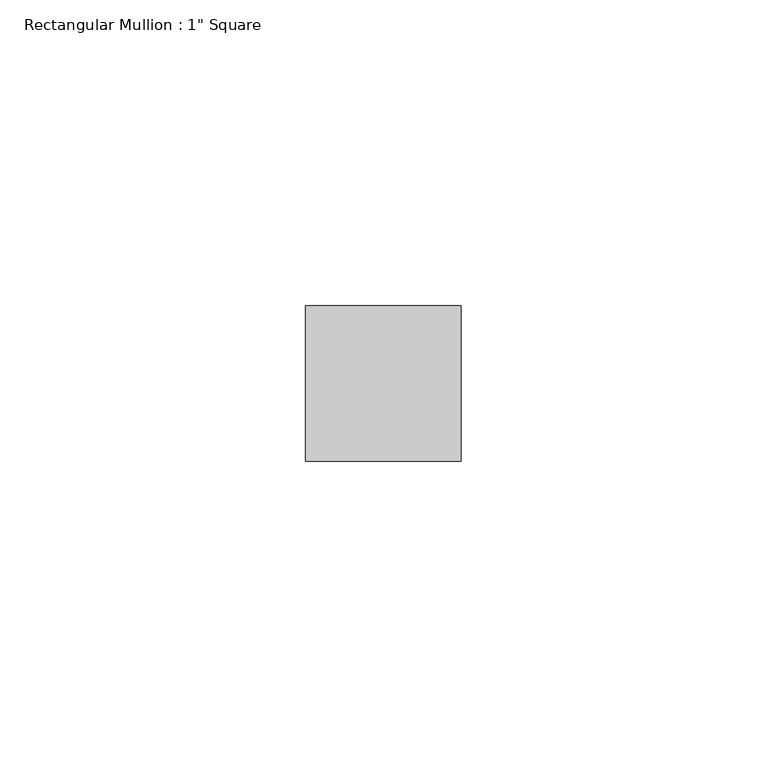
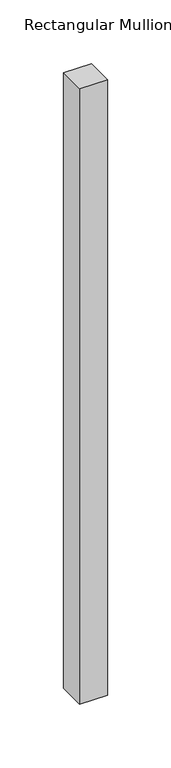
"""IFC4 building model written with IfcOpenShell, lengths in millimetres: member geometry."""

from ifc_helpers import new_model, si_unit, frame, origin, place, context, project, spatial, polyline, outline, extrude, source, transform, mapped, element, save


def member_c698ba88(model_context):
    return source(origin(), model_context, "Body", "SweptSolid", [
        extrude(outline(polyline([(12.7, 12.7), (12.7, -12.7), (-12.7, -12.7), (-12.7, 12.7), (12.7, 12.7)])), frame((0.0, 0.0, -590.55), z_axis=(0.0, 0.0, 1.0), x_axis=(1.0, 0.0, 0.0)), (0.0, 0.0, 1.0), 590.55),
    ])


if __name__ == "__main__":
    model = new_model("IFC4")
    model_context = context("Model", 3, world=origin())
    ifc_project = project(units=[si_unit("LENGTHUNIT", "METRE", prefix="MILLI")], contexts=[model_context])
    site = spatial("IfcSite", under=ifc_project)
    building = spatial("IfcBuilding", under=site)
    placement = place(None, origin())
    member_shape = member_c698ba88(model_context)
    element("IfcMember", 1, ObjectType="Rectangular Mullion : 1\" Square", at=placement, inside=building, context=model_context, shape_type="MappedRepresentation", body=[
        mapped(member_shape, transform((0.0, 0.0, 0.0), x_axis=(1.0, 0.0, 0.0), y_axis=(0.0, 1.0, 0.0), z_axis=(0.0, 0.0, 1.0))),
    ])
    save(model, "model.ifc")

# Revit data of these elements
# Type "Rectangular Mullion : 1\" Square"
#   built-in parameter 1007304 = 0.0833333 (stored number, unit not read)
#   built-in parameter 1007301 = 0.0416667 (stored number, unit not read)
#   built-in parameter 1007300 = 0.0416667 (stored number, unit not read)
